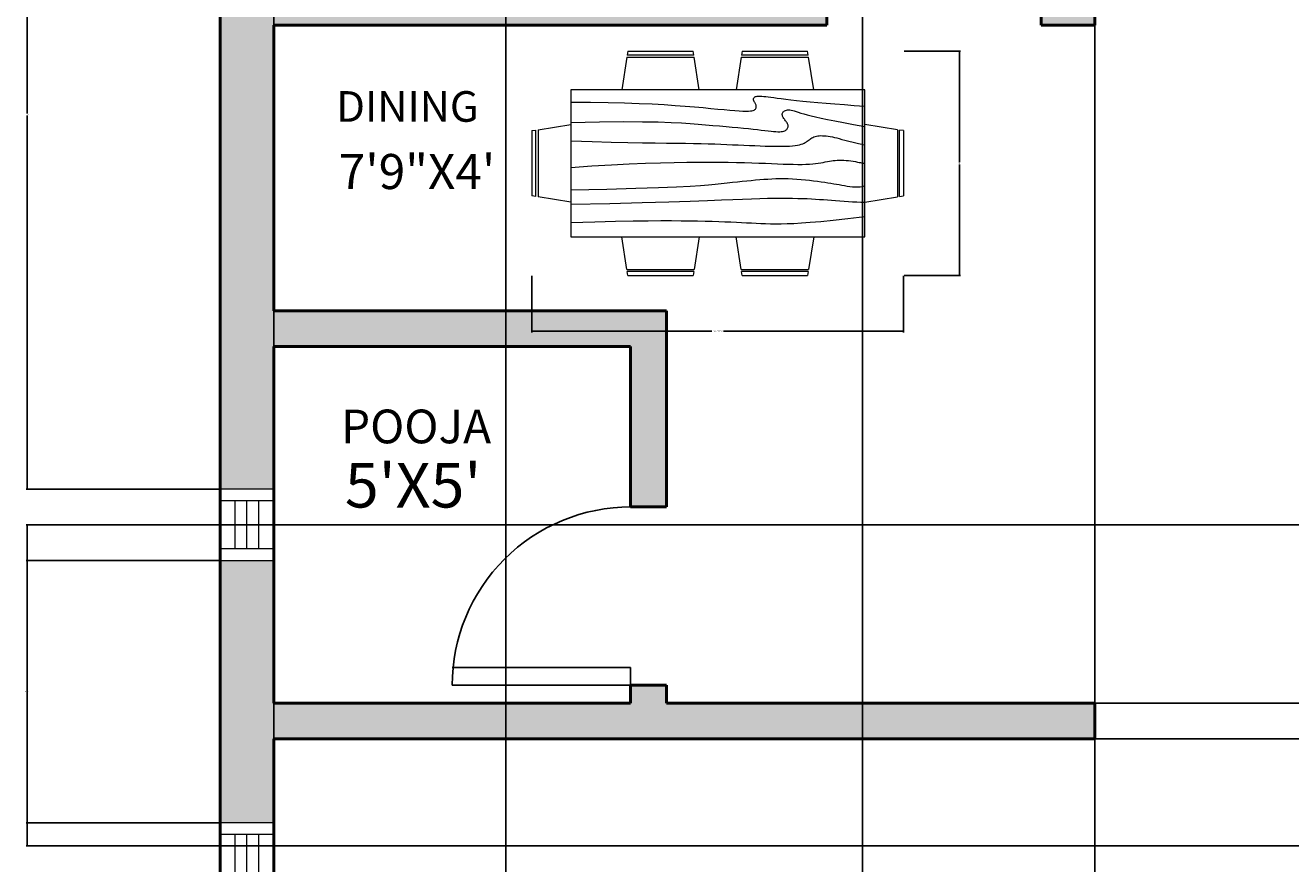
# Model space of a CAD drawing. Units: inches. Extents: x 96 to 522, y 502 to 1213.
# Tile 3 of 5: x 96 to 309, y 856 to 997. Entities that reach past the tile are written whole.
import ezdxf

# ---------------------------------------------------------------- set-up
doc = ezdxf.new("R2010")
doc.units = ezdxf.units.IN
doc.layers.get('Defpoints').update_dxf_attribs({"color": 90})
for name, color, linetype, lineweight in [('A-ANNO-DIMS', 2, 'Continuous', 18), ('A-AREA-IDEN', 7, 'Continuous', 25), ('A-DOOR', 3, 'Continuous', 25), ('A-FURN', 8, 'Continuous', 18), ('A-GLAZ', 4, 'Continuous', 18), ('A-WALL', 7, 'Continuous', 50)]:
    doc.layers.add(name, color=color, linetype=linetype, lineweight=lineweight)
doc.layers.add('A-WALL-PATT', color=252, linetype='Continuous', lineweight=13, true_color=0x939598)
doc.styles.get("Standard").update_dxf_attribs({"font": 'arial.ttf'})
doc.dimstyles.get("Standard").update_dxf_attribs({"dimtxt": 0.18, "dimasz": 0.18, "dimexe": 0.18, "dimexo": 0.0625, "dimgap": 0.09, "dimtad": 0, "dimtih": 1, "dimtoh": 1, "dimdec": 4, "dimzin": 0, "dimdsep": 46, "dimtxsty": 'Standard', "dimcen": 0.09, "dimadec": 0, "dimazin": 0, "dimtfac": 1, "dimtdec": 4, "dimtofl": 0, "dimtmove": 0, "dimatfit": 3, "dimfxl": 1, "dimtolj": 1, "dimtzin": 0, "dimarcsym": 0})

# ---------------------------------------------------------------- blocks, each defined once
blk = doc.blocks.new('Dining Set - 36 x 72 in.')
for p, q in [((-22.2343, 26.00059), (-23.4847, 17.99762)), ((-22.2304, 26), (-5.7608, 26)), ((-22, 27.5), (-22.1562, 26.50042)), ((-5.8416, 26.5), (-22.1534, 26.5)), ((-22, 27.5), (-6, 27.5)), ((-5.8437, 26.49966), (-6, 27.5)), ((-4.5152, 17.99762), (-5.7655, 25.99926)), ((5.7657, 26.00059), (4.5153, 17.99762)), ((5.7696, 26), (22.2392, 26)), ((6, 27.5), (5.8438, 26.50042)), ((22.1584, 26.5), (5.8466, 26.5)), ((6, 27.5), (22, 27.5)), ((22.1563, 26.49966), (22, 27.5)), ((23.4848, 17.99762), (22.2345, 25.99926)), ((36, 18), (-36, 18)), ((-36, 18), (-36, -18)), ((36, -18), (36, 18)), ((-44.0006, 8.23428), (-35.9976, 9.48474)), ((44.0006, 8.23428), (35.9976, 9.48474)), ((-45.5, 8), (-44.5004, 8.15617)), ((-45.5, 8), (-45.5, -8)), ((-44.5, -8.15843), (-44.5, 8.15338)), ((-44, 8.23041), (-44, -8.23915)), ((44, 8.23041), (44, -8.23915)), ((44.5, -8.15843), (44.5, 8.15338)), ((45.5, 8), (44.5005, 8.15617)), ((45.5, 8), (45.5, -8)), ((-44.4997, -8.15631), (-45.5, -8)), ((-35.9976, -9.48476), (-43.9993, -8.2345)), ((35.9976, -9.48476), (43.9993, -8.2345)), ((44.4997, -8.15631), (45.5, -8)), ((-36, -18), (36, -18)), ((-22.2343, -26.0006), (-23.4847, -17.99762)), ((-4.5152, -17.99762), (-5.7655, -25.99928)), ((5.7657, -26.0006), (4.5153, -17.99762)), ((23.4848, -17.99762), (22.2345, -25.99928)), ((-22.2304, -26), (-5.7608, -26)), ((-22, -27.5), (-22.1562, -26.50044)), ((-5.8416, -26.5), (-22.1534, -26.5)), ((-22, -27.5), (-6, -27.5)), ((-5.8437, -26.49967), (-6, -27.5)), ((5.7696, -26), (22.2392, -26)), ((6, -27.5), (5.8438, -26.50044)), ((22.1584, -26.5), (5.8466, -26.5)), ((6, -27.5), (22, -27.5)), ((22.1563, -26.49967), (22, -27.5))]:
    blk.add_line(p, q)
for points in [[(-36, 15), (-31.1772, 14.97754), (-26.8079, 14.91406), (-22.8538, 14.81543), (-19.276, 14.6875), (-16.0362, 14.53613), (-13.0957, 14.36718), (-10.4159, 14.18652), (-7.9583, 14), (-5.6904, 13.81315), (-3.6035, 13.63021), (-1.6954, 13.45508), (0.0365, 13.29166), (1.5945, 13.14388), (2.9811, 13.01562), (4.1988, 12.9108), (5.25, 12.83333), (6.1393, 12.78613), (6.8802, 12.76823), (7.4883, 12.77767), (7.9792, 12.8125), (8.3685, 12.87077), (8.6719, 12.95052), (8.9049, 13.0498), (9.0833, 13.16666), (9.2205, 13.29899), (9.3216, 13.44401), (9.3895, 13.59879), (9.4271, 13.76041), (9.4373, 13.92594), (9.4232, 14.09245), (9.3875, 14.257), (9.3333, 14.41666), (9.2638, 14.56917), (9.1836, 14.71484), (9.0975, 14.85465), (9.0104, 14.98958), (8.9272, 15.1206), (8.8529, 15.2487), (8.7922, 15.37483), (8.75, 15.5), (8.7305, 15.62467), (8.7344, 15.74739), (8.7617, 15.86621), (8.8125, 15.97916), (8.8867, 16.08431), (8.9844, 16.17968), (9.1055, 16.26334), (9.25, 16.33333), (9.4189, 16.38802), (9.6172, 16.42708), (9.8506, 16.45052), (10.125, 16.45833), (10.4463, 16.45052), (10.8203, 16.42708), (11.2529, 16.38802), (11.75, 16.33333), (12.3184, 16.26318), (12.9694, 16.17838), (13.7151, 16.07991), (14.5677, 15.96875), (15.5395, 15.84586), (16.6426, 15.71224), (17.8893, 15.56884), (19.2917, 15.41666), (20.859, 15.25667), (22.5879, 15.08984), (24.4721, 14.91715), (26.5052, 14.73958), (28.6809, 14.5581), (30.9929, 14.3737), (33.4347, 14.18733), (36, 14)], [(-36, 10), (-28.9766, 10.14274), (-23.1725, 10.20442), (-18.4241, 10.19775), (-14.5677, 10.13541), (-11.4399, 10.03011), (-8.877, 9.89453), (-6.7154, 9.74137), (-4.7917, 9.58333), (-2.9698, 9.43082), (-1.2246, 9.28515), (0.4415, 9.14534), (2.026, 9.01041), (3.5266, 8.87939), (4.9408, 8.7513), (6.266, 8.62516), (7.5, 8.5), (8.6411, 8.37549), (9.6914, 8.2539), (10.6538, 8.13818), (11.5312, 8.03125), (12.3267, 7.93603), (13.043, 7.85547), (13.6831, 7.79248), (14.25, 7.75), (14.7471, 7.7303), (15.1797, 7.73307), (15.5537, 7.75732), (15.875, 7.80208), (16.1494, 7.86637), (16.3828, 7.94922), (16.5811, 8.04964), (16.75, 8.16666), (16.8944, 8.29915), (17.0143, 8.44531), (17.1089, 8.60319), (17.1771, 8.77083), (17.218, 8.94629), (17.2305, 9.1276), (17.2137, 9.31282), (17.1667, 9.5), (17.0895, 9.6875), (16.987, 9.875), (16.8649, 10.0625), (16.7292, 10.25), (16.5856, 10.4375), (16.4401, 10.625), (16.2985, 10.8125), (16.1667, 11), (16.05, 11.18733), (15.9518, 11.3737), (15.8752, 11.5581), (15.8229, 11.73958), (15.798, 11.91715), (15.8034, 12.08984), (15.842, 12.25667), (15.9167, 12.41666), (16.0295, 12.56836), (16.1784, 12.70833), (16.3605, 12.83268), (16.5729, 12.9375), (16.8127, 13.01888), (17.0768, 13.07291), (17.3625, 13.0957), (17.6667, 13.08333), (17.9894, 13.03312), (18.3418, 12.94726), (18.7382, 12.82918), (19.1927, 12.68229), (19.7195, 12.51001), (20.3327, 12.31575), (21.0465, 12.10294), (21.875, 11.875), (22.8357, 11.63354), (23.959, 11.37304), (25.2786, 11.08618), (26.8282, 10.76562), (28.6414, 10.40405), (30.752, 9.99414), (33.1936, 9.52856), (36, 9)], [(-36, 5.5), (-30.7157, 5.3348), (-26.069, 5.20963), (-21.9946, 5.11767), (-18.4271, 5.05208), (-15.3009, 5.00602), (-12.5508, 4.97265), (-10.1112, 4.94515), (-7.9167, 4.91666), (-5.909, 4.88167), (-4.0586, 4.83984), (-2.3429, 4.79215), (-0.7396, 4.73958), (0.7739, 4.6831), (2.22, 4.6237), (3.6213, 4.56233), (5, 4.5), (6.373, 4.43782), (7.7344, 4.3776), (9.0723, 4.32129), (10.375, 4.27083), (11.6309, 4.22819), (12.8281, 4.19531), (13.9551, 4.17415), (15, 4.16666), (15.954, 4.17448), (16.819, 4.19791), (17.6001, 4.23698), (18.3021, 4.29166), (18.9299, 4.36198), (19.4883, 4.44791), (19.9823, 4.54948), (20.4167, 4.66666), (20.7969, 4.79899), (21.1302, 4.94401), (21.4245, 5.09879), (21.6875, 5.26041), (21.9271, 5.42594), (22.1511, 5.59245), (22.3672, 5.757), (22.5834, 5.91666), (22.8065, 6.06868), (23.0404, 6.21093), (23.2879, 6.34147), (23.5521, 6.45833), (23.8358, 6.55957), (24.142, 6.64323), (24.4735, 6.70735), (24.8334, 6.75), (25.2235, 6.76969), (25.642, 6.76692), (26.0858, 6.74267), (26.5521, 6.69791), (27.0379, 6.63362), (27.5404, 6.55078), (28.0565, 6.45036), (28.5834, 6.33333), (29.1242, 6.19987), (29.7071, 6.04687), (30.3661, 5.87044), (31.1354, 5.66666), (32.0493, 5.43164), (33.142, 5.16146), (34.4475, 4.85221), (36, 4.5)], [(-36, -1), (-30.7915, -0.6591), (-26.0195, -0.38216), (-21.6519, -0.16284), (-17.6563, 0.00521), (-14.0005, 0.12833), (-10.6523, 0.21289), (-7.5796, 0.26522), (-4.75, 0.29166), (-2.134, 0.29793), (0.2878, 0.28711), (2.5317, 0.26163), (4.6146, 0.22396), (6.5529, 0.17651), (8.3633, 0.12174), (10.0623, 0.06209), (11.6667, 0), (13.1899, -0.06201), (14.6341, -0.1211), (15.9982, -0.17432), (17.2813, -0.21875), (18.4823, -0.25147), (19.6003, -0.26953), (20.6343, -0.27002), (21.5834, -0.25), (22.4481, -0.20768), (23.2357, -0.14584), (23.9549, -0.06836), (24.6146, 0.02083), (25.2235, 0.11784), (25.7904, 0.21875), (26.3241, 0.31966), (26.8334, 0.41666), (27.3265, 0.50618), (27.8099, 0.58593), (28.2894, 0.65397), (28.7709, 0.70833), (29.2601, 0.74707), (29.763, 0.76823), (30.2855, 0.76985), (30.8334, 0.75), (31.4088, 0.70784), (31.9994, 0.64713), (32.589, 0.57275), (33.1615, 0.48958), (33.7008, 0.4025), (34.1908, 0.3164), (34.6153, 0.23616), (34.9584, 0.16666), (35.2099, 0.11165), (35.3848, 0.07031), (35.504, 0.04069), (35.5886, 0.02083), (35.6594, 0.00879), (35.7377, 0.0026), (35.8442, 0.00032), (36, 0)], [(-36, -6.5), (-27.1843, -6.31267), (-20.084, -6.1263), (-14.469, -5.9419), (-10.1094, -5.76042), (-6.7752, -5.58285), (-4.2363, -5.41016), (-2.2629, -5.24333), (-0.625, -5.08334), (0.8708, -4.93099), (2.2715, -4.78646), (3.5872, -4.64974), (4.8281, -4.52084), (6.0046, -4.39974), (7.127, -4.28646), (8.2053, -4.18099), (9.25, -4.08334), (10.2705, -3.99382), (11.2734, -3.91407), (12.2647, -3.84603), (13.25, -3.79167), (14.2354, -3.75293), (15.2266, -3.73177), (16.2295, -3.73015), (17.25, -3.75), (18.2912, -3.79248), (19.3451, -3.85547), (20.4009, -3.93604), (21.4479, -4.03125), (22.4754, -4.13819), (23.4727, -4.25391), (24.4289, -4.37549), (25.3334, -4.5), (26.1785, -4.62492), (26.9694, -4.74935), (27.7145, -4.87281), (28.4219, -4.99479), (29.1, -5.11483), (29.7572, -5.23242), (30.4016, -5.34709), (31.0417, -5.45834), (31.6837, -5.56437), (32.3262, -5.65821), (32.9658, -5.73153), (33.599, -5.77604), (34.2224, -5.78345), (34.8327, -5.74545), (35.4264, -5.65373), (36, -5.5)], [(-36, -10), (-26.4022, -9.81299), (-18.4675, -9.62891), (-11.9839, -9.45069), (-6.7396, -9.28125), (-2.5226, -9.12354), (0.8789, -8.98047), (3.6769, -8.85498), (6.0833, -8.75), (8.2767, -8.66765), (10.3021, -8.60677), (12.1712, -8.56543), (13.8958, -8.54167), (15.4876, -8.53353), (16.9583, -8.53907), (18.3197, -8.55632), (19.5834, -8.58334), (20.7616, -8.61841), (21.8685, -8.66081), (22.9188, -8.71004), (23.9271, -8.76563), (24.9081, -8.82707), (25.8763, -8.89388), (26.8465, -8.96558), (27.8334, -9.04167), (28.8474, -9.12118), (29.8828, -9.20117), (30.93, -9.27824), (31.9792, -9.34896), (33.0205, -9.40991), (34.0443, -9.45768), (35.0407, -9.48885), (36, -9.5)], [(-36, -14.5), (-30.0881, -14.33513), (-25.0332, -14.21224), (-20.7312, -14.12647), (-17.0781, -14.07292), (-13.97, -14.04671), (-11.3027, -14.04297), (-8.9724, -14.05681), (-6.875, -14.08334), (-4.9224, -14.11833), (-3.0905, -14.16016), (-1.3709, -14.20785), (0.2448, -14.26042), (1.7647, -14.3169), (3.1973, -14.3763), (4.5507, -14.43767), (5.8333, -14.5), (7.0554, -14.5621), (8.235, -14.62175), (9.3922, -14.67652), (10.5469, -14.72396), (11.7192, -14.76164), (12.929, -14.78711), (14.1965, -14.79794), (15.5417, -14.79167), (16.9933, -14.76424), (18.6152, -14.70508), (20.4804, -14.60197), (22.6615, -14.44271), (25.2312, -14.21509), (28.2624, -13.9069), (31.8277, -13.50594), (36, -13)]]:
    blk.add_lwpolyline(points)
blk = doc.blocks.new('WIN-60IN')
for p, q in [((60, 9), (0, 9)), ((0, 9), (0, 0)), ((2, 9), (2, 0)), ((58, 0), (58, 9)), ((60, 0), (60, 9)), ((2, 6.5), (58, 6.5)), ((2, 4.5), (58, 4.5)), ((2, 2.5), (58, 2.5)), ((0, 0), (60, 0))]:
    blk.add_line(p, q)
blk = doc.blocks.new('WIN-12IN')
for p, q in [((0, 12), (0, 0)), ((9, 12), (0, 12)), ((9, 0), (9, 12)), ((9, 10), (0, 10)), ((2.5, 10), (2.5, 2)), ((4.5, 10), (4.5, 2)), ((6.5, 10), (6.5, 2)), ((0, 2), (9, 2)), ((0, 0), (9, 0))]:
    blk.add_line(p, q)
blk = doc.blocks.new('DOOR-SGL-30IN')
for p, q in [((30, 30), (0, 30)), ((0, 30), (0, 27)), ((30, 27), (0, 27))]:
    blk.add_line(p, q)
blk.add_arc((0, 30), 30, 270, 0)
blk = doc.blocks.new('*D33')
at = {"layer": 'A-ANNO-DIMS', "color": 0, "lineweight": -2, "transparency": 16777216}
for p, q in [((181.61, 955.1), (181.61, 945.61)), ((244.09, 955.1), (244.09, 945.61)), ((181.79, 945.79), (211.88, 945.79)), ((243.91, 945.79), (213.82, 945.79))]:
    blk.add_line(p, q, dxfattribs=at)
at = {"layer": 'A-ANNO-DIMS', "color": 0, "transparency": 16777216}
for points in [[(181.79, 945.82), (181.79, 945.76), (181.61, 945.79)], [(243.91, 945.82), (243.91, 945.76), (244.09, 945.79)]]:
    blk.add_solid(points, dxfattribs=at)
at = {"layer": 'Defpoints', "color": 0, "transparency": 16777216}
for p in [(181.61, 955.16), (244.09, 955.16), (244.09, 945.79)]:
    blk.add_point(p, dxfattribs=at)
at = {"layer": 'A-ANNO-DIMS', "color": 0, "transparency": 16777216, "insert": (212.85, 945.79), "char_height": 0.18, "attachment_point": 5}
blk.add_mtext('\\A1;DINING SET 62', dxfattribs=at)
blk = doc.blocks.new('*D34')
at = {"layer": 'A-ANNO-DIMS', "color": 0, "lineweight": -2, "transparency": 16777216}
for p, q in [((244.16, 992.92), (253.65, 992.92)), ((253.47, 992.74), (253.47, 974.22)), ((253.47, 955.34), (253.47, 973.86)), ((244.16, 955.16), (253.65, 955.16))]:
    blk.add_line(p, q, dxfattribs=at)
at = {"layer": 'A-ANNO-DIMS', "color": 0, "transparency": 16777216}
for points in [[(253.44, 992.74), (253.5, 992.74), (253.47, 992.92)], [(253.44, 955.34), (253.5, 955.34), (253.47, 955.16)]]:
    blk.add_solid(points, dxfattribs=at)
at = {"layer": 'Defpoints', "color": 0, "transparency": 16777216}
for p in [(244.09, 992.92), (253.47, 992.92), (244.09, 955.16)]:
    blk.add_point(p, dxfattribs=at)
at = {"layer": 'A-ANNO-DIMS', "color": 0, "transparency": 16777216, "insert": (253.47, 974.04), "char_height": 0.18, "attachment_point": 5}
blk.add_mtext('\\A1;38', dxfattribs=at)
blk = doc.blocks.new('*D53')
at = {"layer": 'A-ANNO-DIMS', "color": 0, "lineweight": -2, "transparency": 16777216}
for p, q in [((138.21, 661.31), (138.21, 1212.88)), ((138.39, 1212.7), (157.49, 1212.7)), ((177.03, 1212.7), (157.93, 1212.7)), ((177.21, 661.31), (177.21, 1212.88))]:
    blk.add_line(p, q, dxfattribs=at)
at = {"layer": 'A-ANNO-DIMS', "color": 0, "transparency": 16777216}
for points in [[(138.39, 1212.73), (138.39, 1212.67), (138.21, 1212.7)], [(177.03, 1212.73), (177.03, 1212.67), (177.21, 1212.7)]]:
    blk.add_solid(points, dxfattribs=at)
at = {"layer": 'Defpoints', "color": 0, "transparency": 16777216}
for p in [(177.21, 1212.7), (138.21, 661.25), (177.21, 661.25)]:
    blk.add_point(p, dxfattribs=at)
at = {"layer": 'A-ANNO-DIMS', "color": 0, "transparency": 16777216, "insert": (157.71, 1212.7), "char_height": 0.18, "attachment_point": 5}
blk.add_mtext('\\A1;39', dxfattribs=at)
blk = doc.blocks.new('*D54')
at = {"layer": 'A-ANNO-DIMS', "color": 0, "lineweight": -2, "transparency": 16777216}
for p, q in [((237.21, 661.31), (237.21, 1212.88)), ((237.39, 1212.7), (256.49, 1212.7)), ((276.03, 1212.7), (256.93, 1212.7)), ((276.21, 661.31), (276.21, 1212.88))]:
    blk.add_line(p, q, dxfattribs=at)
at = {"layer": 'A-ANNO-DIMS', "color": 0, "transparency": 16777216}
for points in [[(237.39, 1212.73), (237.39, 1212.67), (237.21, 1212.7)], [(276.03, 1212.73), (276.03, 1212.67), (276.21, 1212.7)]]:
    blk.add_solid(points, dxfattribs=at)
at = {"layer": 'Defpoints', "color": 0, "transparency": 16777216}
for p in [(276.21, 1212.7), (237.21, 661.25), (276.21, 661.25)]:
    blk.add_point(p, dxfattribs=at)
at = {"layer": 'A-ANNO-DIMS', "color": 0, "transparency": 16777216, "insert": (256.71, 1212.7), "char_height": 0.18, "attachment_point": 5}
blk.add_mtext('\\A1;39', dxfattribs=at)
blk = doc.blocks.new('*D58')
at = {"layer": 'A-ANNO-DIMS', "color": 0, "lineweight": -2, "transparency": 16777216}
for p, q in [((129.15, 907.25), (96.58, 907.25)), ((96.76, 907.07), (96.76, 885.38)), ((96.76, 863.32), (96.76, 885.01)), ((129.15, 863.14), (96.58, 863.14))]:
    blk.add_line(p, q, dxfattribs=at)
at = {"layer": 'A-ANNO-DIMS', "color": 0, "transparency": 16777216}
for points in [[(96.73, 907.07), (96.79, 907.07), (96.76, 907.25)], [(96.73, 863.32), (96.79, 863.32), (96.76, 863.14)]]:
    blk.add_solid(points, dxfattribs=at)
at = {"layer": 'Defpoints', "color": 0, "transparency": 16777216}
for p in [(96.76, 907.25), (129.21, 907.25), (129.21, 863.14)]:
    blk.add_point(p, dxfattribs=at)
at = {"layer": 'A-ANNO-DIMS', "color": 0, "transparency": 16777216, "insert": (96.76, 885.2), "char_height": 0.18, "attachment_point": 5}
blk.add_mtext('\\A1;44.11', dxfattribs=at)
blk = doc.blocks.new('*D59')
at = {"layer": 'A-ANNO-DIMS', "color": 0, "lineweight": -2, "transparency": 16777216}
for p, q in [((129.15, 1045.25), (96.58, 1045.25)), ((96.76, 1045.07), (96.76, 982.43)), ((96.76, 919.43), (96.76, 982.07)), ((129.15, 919.25), (96.58, 919.25))]:
    blk.add_line(p, q, dxfattribs=at)
at = {"layer": 'A-ANNO-DIMS', "color": 0, "transparency": 16777216}
for points in [[(96.73, 1045.07), (96.79, 1045.07), (96.76, 1045.25)], [(96.73, 919.43), (96.79, 919.43), (96.76, 919.25)]]:
    blk.add_solid(points, dxfattribs=at)
at = {"layer": 'Defpoints', "color": 0, "transparency": 16777216}
for p in [(96.76, 1045.25), (129.21, 1045.25), (129.21, 919.25)]:
    blk.add_point(p, dxfattribs=at)
at = {"layer": 'A-ANNO-DIMS', "color": 0, "transparency": 16777216, "insert": (96.76, 982.25), "char_height": 0.18, "attachment_point": 5}
blk.add_mtext('\\A1;126', dxfattribs=at)
blk = doc.blocks.new('*D62')
at = {"layer": 'A-ANNO-DIMS', "color": 0, "lineweight": -2, "transparency": 16777216}
for p, q in [((480.15, 913.25), (96.58, 913.25)), ((96.76, 913.07), (96.76, 886.43)), ((96.76, 859.43), (96.76, 886.07)), ((480.15, 859.25), (96.58, 859.25))]:
    blk.add_line(p, q, dxfattribs=at)
at = {"layer": 'A-ANNO-DIMS', "color": 0, "transparency": 16777216}
for points in [[(96.73, 913.07), (96.79, 913.07), (96.76, 913.25)], [(96.73, 859.43), (96.79, 859.43), (96.76, 859.25)]]:
    blk.add_solid(points, dxfattribs=at)
at = {"layer": 'Defpoints', "color": 0, "transparency": 16777216}
for p in [(96.76, 913.25), (480.21, 913.25), (480.21, 859.25)]:
    blk.add_point(p, dxfattribs=at)
at = {"layer": 'A-ANNO-DIMS', "color": 0, "transparency": 16777216, "insert": (96.76, 886.25), "char_height": 0.18, "attachment_point": 5}
blk.add_mtext('\\A1;54', dxfattribs=at)
blk = doc.blocks.new('*D66')
at = {"layer": 'A-ANNO-DIMS', "color": 0, "lineweight": -2, "transparency": 16777216}
for p, q in [((330.21, 1033.19), (330.21, 501.62)), ((276.21, 997.19), (276.21, 501.62)), ((276.39, 501.8), (302.99, 501.8)), ((330.03, 501.8), (303.43, 501.8))]:
    blk.add_line(p, q, dxfattribs=at)
at = {"layer": 'A-ANNO-DIMS', "color": 0, "transparency": 16777216}
for points in [[(276.39, 501.83), (276.39, 501.77), (276.21, 501.8)], [(330.03, 501.83), (330.03, 501.77), (330.21, 501.8)]]:
    blk.add_solid(points, dxfattribs=at)
at = {"layer": 'Defpoints', "color": 0, "transparency": 16777216}
for p in [(330.21, 1033.25), (276.21, 997.25), (330.21, 501.8)]:
    blk.add_point(p, dxfattribs=at)
at = {"layer": 'A-ANNO-DIMS', "color": 0, "transparency": 16777216, "insert": (303.21, 501.8), "char_height": 0.18, "attachment_point": 5}
blk.add_mtext('\\A1;54', dxfattribs=at)
blk = doc.blocks.new('*D67')
at = {"layer": 'A-ANNO-DIMS', "color": 0, "lineweight": -2, "transparency": 16777216}
for p, q in [((276.27, 883.25), (521.84, 883.25)), ((521.66, 883.07), (521.66, 880.43)), ((521.66, 877.43), (521.66, 880.07)), ((276.27, 877.25), (521.84, 877.25))]:
    blk.add_line(p, q, dxfattribs=at)
at = {"layer": 'A-ANNO-DIMS', "color": 0, "transparency": 16777216}
for points in [[(521.63, 883.07), (521.69, 883.07), (521.66, 883.25)], [(521.63, 877.43), (521.69, 877.43), (521.66, 877.25)]]:
    blk.add_solid(points, dxfattribs=at)
at = {"layer": 'Defpoints', "color": 0, "transparency": 16777216}
for p in [(276.21, 883.25), (521.66, 883.25), (276.21, 877.25)]:
    blk.add_point(p, dxfattribs=at)
at = {"layer": 'A-ANNO-DIMS', "color": 0, "transparency": 16777216, "insert": (521.66, 880.25), "char_height": 0.18, "attachment_point": 5}
blk.add_mtext('\\A1;6', dxfattribs=at)

msp = doc.modelspace()

# ---------------------------------------------------------------- hatches: boundary and pattern name
at = {"layer": 'A-WALL-PATT'}
h = msp.add_hatch(color=256, dxfattribs=at)
h.dxf.hatch_style = 1
h.paths.add_polyline_path([(174.2111, 1156.2511), (129.2111, 1156.2511), (129.2111, 1105.2511), (138.2111, 1105.2511), (138.2111, 1147.2511), (174.2111, 1147.2511)])
h.paths.add_polyline_path([(287.2111, 1156.2511), (234.2111, 1156.2511), (234.2111, 1147.2511), (270.2111, 1147.2511), (270.2111, 1003.2511), (267.2111, 1003.2511), (267.2111, 997.2511), (276.2111, 997.2511), (276.2111, 1147.2511), (287.2111, 1147.2511)])
h.paths.add_polyline_path([(342.2111, 1156.2511), (335.2111, 1156.2511), (335.2111, 1147.2511), (338.2111, 1147.2511), (338.2111, 1081.2511), (342.2111, 1081.2511), (342.2111, 1147.2511)])
h.paths.add_polyline_path([(489.2111, 1156.2511), (402.2111, 1156.2511), (402.2111, 1147.2511), (402.2111, 1141.2511), (408.2111, 1141.2511), (408.2111, 1147.2511), (480.2111, 1147.2511), (480.2111, 1123.2511), (489.2111, 1123.2511)])
h.paths.add_polyline_path([(489.2111, 1111.2511), (480.2111, 1111.2511), (480.2111, 1087.2511), (408.2111, 1087.2511), (408.2111, 1111.2511), (402.2111, 1111.2511), (402.2111, 1066.2511), (408.2111, 1066.2511), (408.2111, 1081.2511), (480.2111, 1081.2511), (480.2111, 1063.2511), (489.2111, 1063.2511)])
h.paths.add_polyline_path([(489.2111, 1051.2511), (480.2111, 1051.2511), (480.2111, 1033.2511), (408.2111, 1033.2511), (408.2111, 1036.2511), (402.2111, 1036.2511), (402.2111, 1033.2511), (338.2111, 1033.2511), (330.2111, 1033.2511), (330.2111, 923.2511), (336.2111, 923.2511), (336.2111, 1027.2511), (338.2111, 1027.2511), (402.2111, 1027.2511), (480.2111, 1027.2511), (480.2111, 973.2511), (489.2111, 973.2511)])
h.paths.add_polyline_path([(489.2111, 913.2511), (480.2111, 913.2511), (480.2111, 859.2511), (429.2111, 859.2511), (429.2111, 853.2511), (480.2111, 853.2511), (480.2111, 829.2511), (489.2111, 829.2511)])
h.paths.add_polyline_path([(489.2111, 817.2511), (480.2111, 817.2511), (480.2111, 793.2511), (402.2111, 793.2511), (396.2111, 793.2511), (396.2111, 853.2511), (399.2111, 853.2511), (399.2111, 859.2511), (338.2111, 859.2511), (336.2111, 859.2511), (336.2111, 877.2511), (336.2111, 883.2511), (336.2111, 887.2511), (330.2111, 887.2511), (330.2111, 883.2511), (326.2111, 883.2511), (326.2111, 877.2511), (330.2111, 877.2511), (330.2111, 853.2511), (338.2111, 853.2511), (390.2111, 853.2511), (390.2111, 793.2511), (387.2111, 793.2511), (387.2111, 787.2511), (402.2111, 787.2511), (480.2111, 787.2511), (480.2111, 754.2511), (489.2111, 754.2511)])
h.paths.add_polyline_path([(489.2111, 694.2511), (480.2111, 694.2511), (480.2111, 661.2511), (432.2111, 661.2511), (432.2111, 652.2511), (480.2111, 652.2511), (480.2111, 543.2511), (333.2111, 543.2511), (333.2111, 534.2511), (489.2111, 534.2511), (489.2111, 652.2511)])
h.paths.add_polyline_path([(372.2111, 661.2511), (336.2111, 661.2511), (336.2111, 787.2511), (338.2111, 787.2511), (351.2111, 787.2511), (351.2111, 793.2511), (338.2111, 793.2511), (330.2111, 793.2511), (330.2111, 661.2511), (324.2111, 661.2511), (324.2111, 652.2511), (372.2111, 652.2511)])
h.paths.add_polyline_path([(138.2111, 680.6946), (129.2111, 680.6946), (129.2111, 652.2511), (177.2111, 652.2511), (177.2111, 661.2511), (138.2111, 661.2511)])
h.paths.add_polyline_path([(276.2111, 661.2511), (237.2111, 661.2511), (237.2111, 652.2511), (276.2111, 652.2511)])
h.paths.add_polyline_path([(138.2111, 803.1393), (129.2111, 803.1393), (129.2111, 740.6946), (138.2111, 740.6946)])
h.paths.add_polyline_path([(138.2111, 907.2511), (129.2111, 907.2511), (129.2111, 863.1393), (138.2111, 863.1393), (138.2111, 877.2511), (276.2111, 877.2511), (276.2111, 883.2511), (204.2111, 883.2511), (204.2111, 886.2511), (198.2111, 886.2511), (198.2111, 883.2511), (138.2111, 883.2511)])
h.paths.add_polyline_path([(138.2111, 943.2511), (198.2111, 943.2511), (198.2111, 916.2511), (204.2111, 916.2511), (204.2111, 949.2511), (138.2111, 949.2511), (138.2111, 997.2511), (231.2111, 997.2511), (231.2111, 1003.2511), (138.2111, 1003.2511), (138.2111, 1045.2511), (129.2111, 1045.2511), (129.2111, 919.2511), (138.2111, 919.2511)])

# ---------------------------------------------------------------- linework, layer by layer
at = {"layer": 'A-WALL'}
for p, q in [((276.2111, 1147.2511), (276.2111, 997.2511)), ((231.2111, 1003.2511), (231.2111, 997.2511)), ((267.2111, 1003.2511), (267.2111, 997.2511)), ((231.2111, 997.2511), (138.2111, 997.2511)), ((138.2111, 997.2511), (138.2111, 949.2511)), ((276.2111, 997.2511), (267.2111, 997.2511)), ((204.2111, 949.2511), (138.2111, 949.2511)), ((204.2111, 949.2511), (204.2111, 916.2511)), ((198.2111, 943.2511), (138.2111, 943.2511)), ((138.2111, 943.2511), (138.2111, 883.2511)), ((198.2111, 943.2511), (198.2111, 916.2511)), ((204.2111, 916.2511), (198.2111, 916.2511)), ((204.2111, 886.2511), (198.2111, 886.2511)), ((198.2111, 886.2511), (198.2111, 883.2511)), ((204.2111, 886.2511), (204.2111, 883.2511)), ((198.2111, 883.2511), (138.2111, 883.2511)), ((276.2111, 883.2511), (204.2111, 883.2511)), ((276.2111, 883.2511), (276.2111, 877.2511)), ((276.2111, 877.2511), (138.2111, 877.2511)), ((138.2111, 877.2511), (138.2111, 661.2511))]:
    msp.add_line(p, q, dxfattribs=at)
msp.add_lwpolyline([(287.2111, 1156.2511), (129.2111, 1156.2511), (129.2111, 652.2511), (276.2111, 652.2511)], dxfattribs=at)

# ---------------------------------------------------------------- block references
at = {"layer": 'A-DOOR', "rotation": 180}
msp.add_blockref('DOOR-SGL-30IN', (198.2111, 916.2511), dxfattribs=at)
at = {"layer": 'A-FURN', "xscale": 0.6865992929511716, "yscale": 0.6865992929511716, "zscale": 0.6865992929511716}
msp.add_blockref('Dining Set - 36 x 72 in.', (212.8527, 974.0417), dxfattribs=at)
at = {"layer": 'A-GLAZ'}
for name, p, rotation in [('WIN-12IN', (138.2111, 919.2511), 180), ('WIN-60IN', (138.2111, 803.1393), 89.99999999999984)]:
    msp.add_blockref(name, p, dxfattribs=dict(at, rotation=rotation))

# ---------------------------------------------------------------- texts
at = {"layer": 'A-AREA-IDEN', "attachment_point": 1}
for s, width, gutter_width, insert, char_height in [('DINING', 28.223042, 25.7345, (148.7246, 986.1749), 5.1469), ('7\'9"X4\'', 32.350385, 29.4979, (149.1487, 975.6061), 5.89959), ('POOJA', 31.119044, 28.3752, (149.5198, 932.6238), 5.67503), ("5'X5'", 41.174278, 37.5438, (150.1772, 923.6636), 7.50876)]:
    msp.add_mtext_dynamic_manual_height_columns(s, width=width, gutter_width=gutter_width, heights=[0], dxfattribs=dict(at, insert=insert, char_height=char_height))

# ---------------------------------------------------------------- dimensions: what is measured, and where the dimension line sits
at = {"layer": 'A-ANNO-DIMS'}
for base, p1, p2, picture, middle in [((177.2111, 1212.7011), (138.2111, 661.2511), (177.2111, 661.2511), '*D53', (157.7111, 1212.7011)), ((276.2111, 1212.7011), (237.2111, 661.2511), (276.2111, 661.2511), '*D54', (256.7111, 1212.7011)), ((330.2111, 501.8011), (276.2111, 997.2511), (330.2111, 1033.2511), '*D66', (303.2111, 501.8011))]:
    dim = msp.add_linear_dim(base=base, p1=p1, p2=p2, dimstyle='Standard', override={"dimdec": 0, "dimlfac": 1, "dimrnd": 0, "dimzin": 0, "dimdsep": 46, "dimlunit": 2}, dxfattribs=at)
    dim.commit()
    dim.dimension.update_dxf_attribs({"geometry": picture, "text_midpoint": middle})
for base, p1, p2, override, picture, middle in [((96.7611, 1045.2511), (129.2111, 919.2511), (129.2111, 1045.2511), {"dimdec": 0, "dimlfac": 1, "dimrnd": 0, "dimzin": 0, "dimdsep": 46, "dimlunit": 2}, '*D59', (96.7611, 982.2511)), ((253.465, 992.9232), (244.0929, 955.1602), (244.0929, 992.9232), {"dimdec": 0, "dimlfac": 1, "dimrnd": 0, "dimzin": 0, "dimdsep": 46, "dimlunit": 2}, '*D34', (253.465, 974.0417)), ((96.7611, 913.2511), (480.2111, 859.2511), (480.2111, 913.2511), {"dimdec": 0, "dimlfac": 1, "dimrnd": 0, "dimzin": 0, "dimdsep": 46, "dimlunit": 2}, '*D62', (96.7611, 886.2511)), ((96.7611, 907.2511), (129.2111, 863.1393), (129.2111, 907.2511), {"dimdec": 2, "dimlfac": 1, "dimrnd": 0, "dimzin": 0, "dimdsep": 46, "dimlunit": 2}, '*D58', (96.7611, 885.1952)), ((521.6611, 883.2511), (276.2111, 877.2511), (276.2111, 883.2511), {"dimdec": 0, "dimlfac": 1, "dimrnd": 0, "dimzin": 0, "dimdsep": 46, "dimlunit": 2}, '*D67', (521.6611, 880.2511))]:
    dim = msp.add_linear_dim(base=base, p1=p1, p2=p2, angle=90, dimstyle='Standard', override=override, dxfattribs=at)
    dim.commit()
    dim.dimension.update_dxf_attribs({"geometry": picture, "text_midpoint": middle})
dim = msp.add_linear_dim(base=(244.0929, 945.7881), p1=(181.6124, 955.1602), p2=(244.0929, 955.1602), text='DINING SET <>', dimstyle='Standard', override={"dimdec": 0, "dimlfac": 1, "dimrnd": 0, "dimzin": 0, "dimdsep": 46, "dimlunit": 2}, dxfattribs=at)
dim.commit()
dim.dimension.update_dxf_attribs({"geometry": '*D33', "text_midpoint": (212.8527, 945.7881)})

doc.saveas('drawing.dxf')
